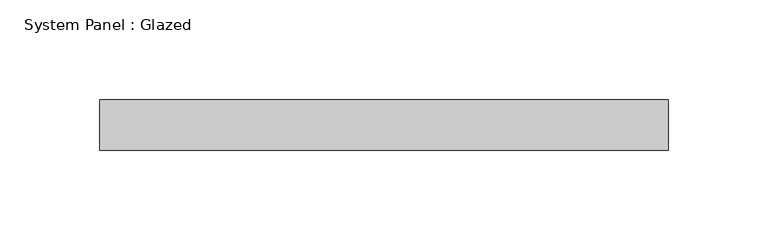
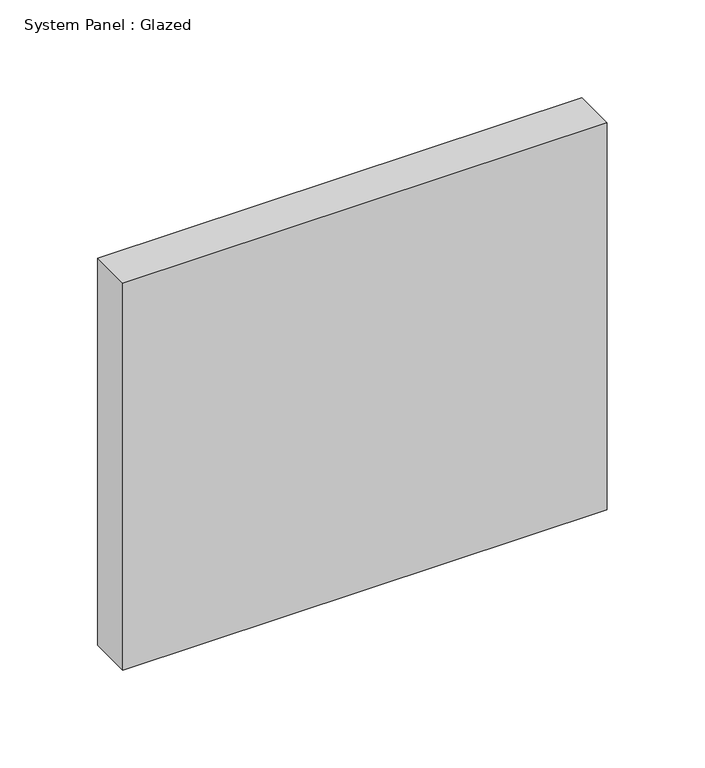
"""IFC4 building model written with IfcOpenShell, lengths in millimetres: plate geometry, System Panel : Glazed."""

from ifc_helpers import new_model, si_unit, origin, origin_with_axes, place, context, project, spatial, polyline, outline, extrude, source, transform, mapped, element, save


def system_panel_glazed_5768b914(model_context):
    return source(origin(), model_context, "Body", "SweptSolid", [
        extrude(outline(polyline([(142.875, 19.05), (-142.875, 19.05), (-142.875, 44.45), (142.875, 44.45), (142.875, 19.05)])), origin_with_axes(), (0.0, 0.0, 1.0), 241.3),
    ])


if __name__ == "__main__":
    model = new_model("IFC4")
    model_context = context("Model", 3, world=origin())
    ifc_project = project(units=[si_unit("LENGTHUNIT", "METRE", prefix="MILLI")], contexts=[model_context])
    site = spatial("IfcSite", under=ifc_project)
    building = spatial("IfcBuilding", under=site)
    placement = place(None, origin())
    system_panel_glazed_shape = system_panel_glazed_5768b914(model_context)
    element("IfcPlate", 1, ObjectType="System Panel : Glazed", at=placement, inside=building, context=model_context, shape_type="MappedRepresentation", body=[
        mapped(system_panel_glazed_shape, transform((0.0, 0.0, 0.0), x_axis=(1.0, 0.0, 0.0), y_axis=(0.0, 1.0, 0.0), z_axis=(0.0, 0.0, 1.0))),
    ])
    save(model, "model.ifc")

# Revit data of these elements
# Type "System Panel : Glazed"
#   Construction Type Id = "GSP4R"
#   Analytic Construction = "1/8 in Pilkington single glazing"
#   Visual Light Transmittance = 0.9
#   Solar Heat Gain Coefficient = 0.86
#   Heat Transfer Coefficient (U) = 1.18115 BTU/(h·ft²·°F)
#   Define Thermal Properties by = 1
# Element 1 (IfcPlate, "System Panel : Glazed")
#   Materials on its faces: "Glass"
# Materials
#   "Glass": class "Glass", colour RGB 0 128 192, transparency 0.75, Description = "Soda Lime Glass", Cost = 0
